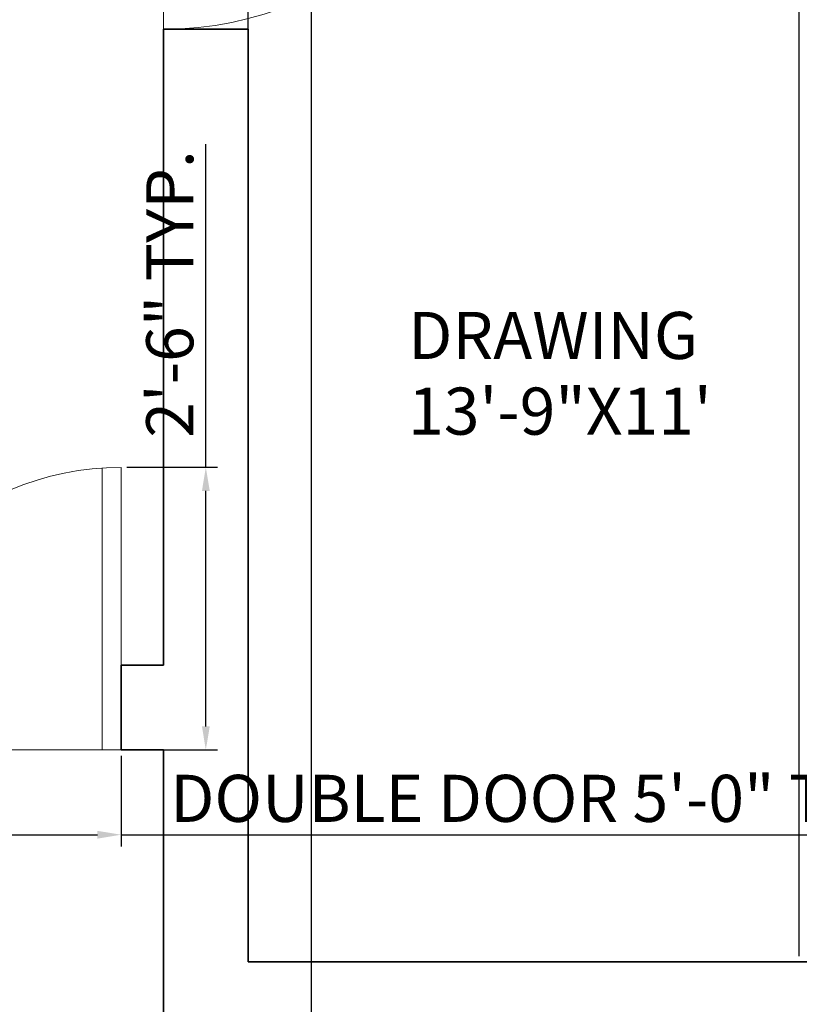
# Model space of a CAD drawing. Units: inches. Extents: x 1265 to 2734, y 1741 to 2595.
# Tile 4 of 10: x 2490 to 2573, y 1988 to 2092. Entities that reach past the tile are written whole.
import ezdxf

# ---------------------------------------------------------------- set-up
doc = ezdxf.new("R2010")
doc.units = ezdxf.units.IN
doc.header["$LTSCALE"] = 0.1
for name, color, linetype, lineweight in [('A-ANNO-DIMS', 2, 'Continuous', 18), ('A-AREA-IDEN', 7, 'Continuous', 18), ('A-DOOR', 3, 'Continuous', 18), ('A-WALL', 7, 'Continuous', 35)]:
    doc.layers.add(name, color=color, linetype=linetype, lineweight=lineweight)
doc.styles.get("Standard").update_dxf_attribs({"font": 'arial.ttf', "height": 5})
doc.dimstyles.new('ISO-25', dxfattribs={"dimtxt": 5, "dimasz": 2.5, "dimexe": 1.25, "dimexo": 0.625, "dimtad": 1, "dimlunit": 3, "dimtxsty": 'Standard', "dimcen": 2.5, "dimadec": 0, "dimazin": 0, "dimtfac": 1, "dimtmove": 0, "dimatfit": 3, "dimfxl": 1, "dimarcsym": 0})

# ---------------------------------------------------------------- blocks, each defined once
blk = doc.blocks.new('DOOR-SWING-36IN')
for p, q in [((33.6, 35.92), (33.6, 0)), ((36, 36), (36, 0)), ((36, 0), (0, 0))]:
    blk.add_line(p, q)
blk.add_arc((36, 0), 36, 90, 180)
blk = doc.blocks.new('DOOR-PAIR-60IN')
for p, q in [((0, 30), (0, 0)), ((2, 29.93), (2, 0)), ((58, 29.93), (58, 0)), ((60, 30), (60, 0)), ((0, 0), (30, 0)), ((60, 0), (30, 0))]:
    blk.add_line(p, q)
for centre, start, end in [((0, 0), 0, 90), ((60, 0), 90, 180)]:
    blk.add_arc(centre, 30, start, end)
blk = doc.blocks.new('*D34')
at = {"layer": 'A-ANNO-DIMS', "color": 0, "lineweight": -2, "transparency": 16777216}
for p, q in [((2441.1, 2014.03), (2441.1, 2004.41)), ((2501.1, 2014.03), (2501.1, 2004.41)), ((2443.6, 2005.66), (2498.6, 2005.66)), ((2501.1, 2005.66), (2588.64, 2005.66))]:
    blk.add_line(p, q, dxfattribs=at)
at = {"layer": 'A-ANNO-DIMS', "color": 0, "lineweight": 100, "transparency": 16777216}
for points in [[(2443.6, 2006.07), (2443.6, 2005.24), (2441.1, 2005.66)], [(2498.6, 2006.07), (2498.6, 2005.24), (2501.1, 2005.66)]]:
    blk.add_solid(points, dxfattribs=at)
at = {"layer": 'Defpoints', "color": 0, "lineweight": 100, "transparency": 16777216}
for p in [(2441.1, 2014.66), (2501.1, 2014.66), (2501.1, 2005.66)]:
    blk.add_point(p, dxfattribs=at)
at = {"layer": 'A-ANNO-DIMS', "color": 0, "transparency": 16777216, "insert": (2546.12, 2008.87), "char_height": 5, "attachment_point": 5}
blk.add_mtext('DOUBLE DOOR 5\'-0" TYP.', dxfattribs=at)
blk = doc.blocks.new('*D35')
at = {"layer": 'A-ANNO-DIMS', "color": 0, "lineweight": -2, "transparency": 16777216}
for p, q in [((2510.1, 2044.66), (2510.1, 2078.97)), ((2501.73, 2044.66), (2511.35, 2044.66)), ((2510.1, 2017.16), (2510.1, 2042.16)), ((2501.73, 2014.66), (2511.35, 2014.66))]:
    blk.add_line(p, q, dxfattribs=at)
at = {"layer": 'A-ANNO-DIMS', "color": 0, "lineweight": 100, "transparency": 16777216}
for points in [[(2509.69, 2042.16), (2510.52, 2042.16), (2510.1, 2044.66)], [(2509.69, 2017.16), (2510.52, 2017.16), (2510.1, 2014.66)]]:
    blk.add_solid(points, dxfattribs=at)
at = {"layer": 'Defpoints', "color": 0, "lineweight": 100, "transparency": 16777216}
for p in [(2501.1, 2044.66), (2510.1, 2044.66), (2501.1, 2014.66)]:
    blk.add_point(p, dxfattribs=at)
at = {"layer": 'A-ANNO-DIMS', "color": 0, "transparency": 16777216, "insert": (2506.92, 2063.06), "char_height": 5, "attachment_point": 5, "rotation": 90}
blk.add_mtext('2\'-6" TYP.', dxfattribs=at)
blk = doc.blocks.new('*D41')
at = {"layer": 'A-ANNO-DIMS', "color": 0, "lineweight": -2, "transparency": 16777216}
for p, q in [((2336.98, 2014.66), (2286.1, 2014.66)), ((2287.35, 2012.16), (2287.35, 1985.66)), ((2504.98, 1983.16), (2286.1, 1983.16))]:
    blk.add_line(p, q, dxfattribs=at)
at = {"layer": 'A-ANNO-DIMS', "color": 0, "lineweight": 100, "transparency": 16777216}
for points in [[(2286.94, 2012.16), (2287.77, 2012.16), (2287.35, 2014.66)], [(2286.94, 1985.66), (2287.77, 1985.66), (2287.35, 1983.16)]]:
    blk.add_solid(points, dxfattribs=at)
at = {"layer": 'Defpoints', "color": 0, "lineweight": 100, "transparency": 16777216}
for p in [(2337.6, 2014.66), (2287.35, 1983.16), (2505.6, 1983.16)]:
    blk.add_point(p, dxfattribs=at)
at = {"layer": 'A-ANNO-DIMS', "color": 0, "transparency": 16777216, "insert": (2284.14, 1998.91), "char_height": 5, "attachment_point": 5, "rotation": 90}
blk.add_mtext('2\'-7 1/2"', dxfattribs=at)
blk = doc.blocks.new('*D42')
at = {"layer": 'A-ANNO-DIMS', "color": 0, "lineweight": -2, "transparency": 16777216}
for p, q in [((2328.6, 1822.68), (2328.6, 2585.16)), ((2521.32, 1822.68), (2521.32, 2585.16)), ((2331.1, 2583.91), (2518.82, 2583.91))]:
    blk.add_line(p, q, dxfattribs=at)
at = {"layer": 'A-ANNO-DIMS', "color": 0, "lineweight": 100, "transparency": 16777216}
for points in [[(2331.1, 2584.32), (2331.1, 2583.49), (2328.6, 2583.91)], [(2518.82, 2584.32), (2518.82, 2583.49), (2521.32, 2583.91)]]:
    blk.add_solid(points, dxfattribs=at)
at = {"layer": 'Defpoints', "color": 0, "lineweight": 100, "transparency": 16777216}
for p in [(2521.32, 2583.91), (2328.6, 1822.06), (2521.32, 1822.06)]:
    blk.add_point(p, dxfattribs=at)
at = {"layer": 'A-ANNO-DIMS', "color": 0, "transparency": 16777216, "insert": (2424.96, 2587.12), "char_height": 5, "attachment_point": 5}
blk.add_mtext('16\'-0 1/2"', dxfattribs=at)
blk = doc.blocks.new('*D47')
at = {"layer": 'A-ANNO-DIMS', "color": 0, "lineweight": -2, "transparency": 16777216}
for p, q in [((2514.6, 1992.78), (2514.6, 2585.16)), ((2573.1, 1992.78), (2573.1, 2585.16)), ((2517.1, 2583.91), (2570.6, 2583.91))]:
    blk.add_line(p, q, dxfattribs=at)
at = {"layer": 'A-ANNO-DIMS', "color": 0, "lineweight": 100, "transparency": 16777216}
for points in [[(2517.1, 2584.32), (2517.1, 2583.49), (2514.6, 2583.91)], [(2570.6, 2584.32), (2570.6, 2583.49), (2573.1, 2583.91)]]:
    blk.add_solid(points, dxfattribs=at)
at = {"layer": 'Defpoints', "color": 0, "lineweight": 100, "transparency": 16777216}
for p in [(2573.1, 2583.91), (2514.6, 1992.16), (2573.1, 1992.16)]:
    blk.add_point(p, dxfattribs=at)
at = {"layer": 'A-ANNO-DIMS', "color": 0, "transparency": 16777216, "insert": (2543.85, 2587.12), "char_height": 5, "attachment_point": 5}
blk.add_mtext('4\'-10 1/2"', dxfattribs=at)

msp = doc.modelspace()

# ---------------------------------------------------------------- linework, layer by layer
at = {"layer": 'A-WALL'}
for p, q in [((2505.602, 2023.657), (2505.602, 2091.157)), ((2505.602, 2091.157), (2514.602, 2091.157)), ((2514.602, 1992.157), (2514.602, 2091.157)), ((2501.102, 2023.657), (2501.102, 2014.657)), ((2501.102, 2023.657), (2505.602, 2023.657)), ((2501.102, 2014.657), (2505.602, 2014.657)), ((2505.602, 1983.157), (2505.602, 2014.657)), ((2514.602, 1992.157), (2679.602, 1992.157))]:
    msp.add_line(p, q, dxfattribs=at)

# ---------------------------------------------------------------- block references
at = {"layer": 'A-DOOR', "extrusion": (0, 0, -1), "zscale": -1, "rotation": 90.0000000000019}
msp.add_blockref('DOOR-SWING-36IN', (-2505.603, 2091.156), dxfattribs=at)
at = {"layer": 'A-DOOR'}
msp.add_blockref('DOOR-PAIR-60IN', (2441.103, 2014.657), dxfattribs=at)

# ---------------------------------------------------------------- texts
at = {"layer": 'A-AREA-IDEN'}
for s, p in [('DRAWING', (2531.582, 2056.156)), ('13\'-9"X11\'', (2531.582, 2048.124))]:
    msp.add_text(s, height=5, dxfattribs=at).set_placement(p)

# ---------------------------------------------------------------- dimensions: what is measured, and where the dimension line sits
at = {"layer": 'A-ANNO-DIMS'}
for base, p1, p2, picture, middle in [((2521.319, 2583.907), (2328.602, 1822.059), (2521.319, 1822.059), '*D42', (2424.961, 2587.117)), ((2573.102, 2583.907), (2514.602, 1992.157), (2573.102, 1992.157), '*D47', (2543.852, 2587.117))]:
    dim = msp.add_linear_dim(base=base, p1=p1, p2=p2, dimstyle='ISO-25', override={"dimdec": 1, "dimlfac": 1, "dimrnd": 0, "dimzin": 1, "dimdsep": 46, "dimlunit": 4, "dimfrac": 2}, dxfattribs=at)
    dim.commit()
    dim.dimension.update_dxf_attribs({"geometry": picture, "text_midpoint": middle})
dim = msp.add_linear_dim(base=(2510.102, 2044.657), p1=(2501.102, 2014.657), p2=(2501.102, 2044.657), angle=90, text='<> TYP.', dimstyle='ISO-25', override={"dimdec": 1, "dimlfac": 1, "dimrnd": 0, "dimzin": 1, "dimdsep": 46, "dimlunit": 4, "dimfrac": 2}, dxfattribs=at)
dim.commit()
dim.dimension.update_dxf_attribs({"geometry": '*D35', "text_midpoint": (2506.925, 2063.063)})
dim = msp.add_linear_dim(base=(2501.102, 2005.657), p1=(2441.102, 2014.657), p2=(2501.102, 2014.657), text='DOUBLE DOOR <> TYP.', dimstyle='ISO-25', override={"dimdec": 1, "dimlfac": 1, "dimrnd": 0, "dimzin": 1, "dimdsep": 46, "dimlunit": 4, "dimfrac": 2}, dxfattribs=at)
dim.commit()
dim.dimension.update_dxf_attribs({"geometry": '*D34', "text_midpoint": (2546.122, 2008.869)})
dim = msp.add_linear_dim(base=(2287.352, 1983.157), p1=(2337.602, 2014.657), p2=(2505.602, 1983.157), angle=90, dimstyle='ISO-25', override={"dimdec": 1, "dimlfac": 1, "dimrnd": 0, "dimzin": 1, "dimdsep": 46, "dimlunit": 4, "dimfrac": 2}, dxfattribs=at)
dim.commit()
dim.dimension.update_dxf_attribs({"geometry": '*D41', "text_midpoint": (2284.142, 1998.907)})

doc.saveas('drawing.dxf')
